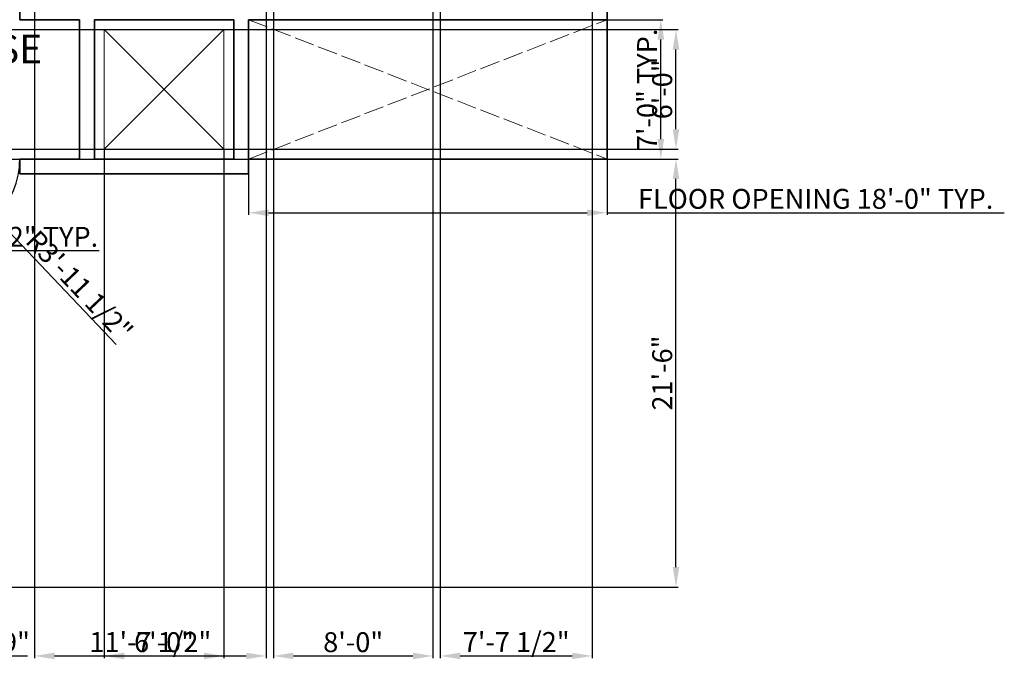
# Model space of a CAD drawing. Units: inches. Extents: x 2174 to 3353, y 1481 to 2316.
# Tile 6 of 8: x 2759 to 3353, y 1501 to 1896. Entities that reach past the tile are written whole.
import ezdxf

# ---------------------------------------------------------------- set-up
doc = ezdxf.new("R2010")
doc.units = ezdxf.units.IN
doc.linetypes.add('ACAD_ISO02W100', pattern=[15, 12, -3])
for name, color, linetype, lineweight in [('A-ANNO-DIMS', 2, 'Continuous', 18), ('A-AREA-IDEN', 7, 'Continuous', 25), ('A-DOOR', 4, 'Continuous', 25), ('A-FLOR-OPEN', 8, 'ACAD_ISO02W100', 13), ('A-FLOR-SHFT', 8, 'Continuous', 18), ('A-WALL', 7, 'Continuous', 35)]:
    doc.layers.add(name, color=color, linetype=linetype, lineweight=lineweight)
doc.styles.get("Standard").update_dxf_attribs({"font": 'arial.ttf'})
doc.dimstyles.new('ISO-25', dxfattribs={"dimtxt": 12, "dimasz": 12, "dimexe": 1.25, "dimexo": 0.625, "dimtad": 1, "dimlunit": 3, "dimtxsty": 'Standard', "dimcen": 2.5, "dimadec": 0, "dimazin": 0, "dimtfac": 1, "dimtmove": 0, "dimatfit": 3, "dimfxl": 1, "dimarcsym": 0})

# ---------------------------------------------------------------- blocks, each defined once
blk = doc.blocks.new('OPENING-CROSS-18FT-7FT')
for p, q in [((0, 0), (216, 84)), ((0, 84), (216, 0))]:
    blk.add_line(p, q)
blk = doc.blocks.new('*D24')
at = {"layer": 'A-ANNO-DIMS', "color": 0, "lineweight": -2, "transparency": 16777216}
for p, q in [((2706.94, 1762.98), (2706.94, 1755.16)), ((2708.94, 1762.98), (2708.94, 1755.16)), ((2694.94, 1756.41), (2682.94, 1756.41)), ((2706.94, 1756.41), (2708.94, 1756.41)), ((2720.94, 1756.41), (2807.34, 1756.41))]:
    blk.add_line(p, q, dxfattribs=at)
at = {"layer": 'A-ANNO-DIMS', "color": 0, "transparency": 16777216}
for points in [[(2694.94, 1758.41), (2694.94, 1754.41), (2706.94, 1756.41)], [(2720.94, 1758.41), (2720.94, 1754.41), (2708.94, 1756.41)]]:
    blk.add_solid(points, dxfattribs=at)
at = {"layer": 'Defpoints', "color": 0, "transparency": 16777216}
for p in [(2706.94, 1763.61), (2708.94, 1763.61), (2708.94, 1756.41)]:
    blk.add_point(p, dxfattribs=at)
at = {"layer": 'A-ANNO-DIMS', "color": 0, "transparency": 16777216, "insert": (2770.14, 1763.16), "char_height": 12, "attachment_point": 5}
blk.add_mtext('0\'-2" TYP.', dxfattribs=at)
blk = doc.blocks.new('*D31')
at = {"layer": 'A-ANNO-DIMS', "color": 0, "lineweight": -2, "transparency": 16777216}
for p, q in [((2916.37, 1919.69), (2916.37, 1908.31)), ((2988.05, 1919.69), (2988.05, 1908.31)), ((2928.37, 1909.56), (2976.05, 1909.56)), ((2988.05, 1909.56), (3211.72, 1909.56))]:
    blk.add_line(p, q, dxfattribs=at)
at = {"layer": 'A-ANNO-DIMS', "color": 0, "transparency": 16777216}
for points in [[(2928.37, 1911.56), (2928.37, 1907.56), (2916.37, 1909.56)], [(2976.05, 1911.56), (2976.05, 1907.56), (2988.05, 1909.56)]]:
    blk.add_solid(points, dxfattribs=at)
at = {"layer": 'Defpoints', "color": 0, "transparency": 16777216}
for p in [(2916.37, 1920.31), (2988.05, 1920.31), (2988.05, 1909.56)]:
    blk.add_point(p, dxfattribs=at)
at = {"layer": 'A-ANNO-DIMS', "color": 0, "transparency": 16777216, "insert": (3105.88, 1916.39), "char_height": 12, "attachment_point": 5}
blk.add_mtext('DINING SET 5\'-11 1/2" TYP.', dxfattribs=at)
blk = doc.blocks.new('*D39')
at = {"layer": 'A-ANNO-DIMS', "color": 0, "lineweight": -2, "transparency": 16777216}
for p, q in [((2897.44, 1810.98), (2897.44, 1777.96)), ((3113.44, 1810.98), (3113.44, 1777.96)), ((2909.44, 1779.21), (3101.44, 1779.21)), ((3113.44, 1779.21), (3352.86, 1779.21))]:
    blk.add_line(p, q, dxfattribs=at)
at = {"layer": 'A-ANNO-DIMS', "color": 0, "transparency": 16777216}
for points in [[(2909.44, 1781.21), (2909.44, 1777.21), (2897.44, 1779.21)], [(3101.44, 1781.21), (3101.44, 1777.21), (3113.44, 1779.21)]]:
    blk.add_solid(points, dxfattribs=at)
at = {"layer": 'Defpoints', "color": 0, "transparency": 16777216}
for p in [(2897.44, 1811.61), (3113.44, 1811.61), (3113.44, 1779.21)]:
    blk.add_point(p, dxfattribs=at)
at = {"layer": 'A-ANNO-DIMS', "color": 0, "transparency": 16777216, "insert": (3239.15, 1786.04), "char_height": 12, "attachment_point": 5}
blk.add_mtext('FLOOR OPENING 18\'-0" TYP.', dxfattribs=at)
blk = doc.blocks.new('*D40')
at = {"layer": 'A-ANNO-DIMS', "color": 0, "lineweight": -2, "transparency": 16777216}
for p, q in [((3114.07, 1895.61), (3147.09, 1895.61)), ((3145.84, 1823.61), (3145.84, 1883.61)), ((3114.07, 1811.61), (3147.09, 1811.61))]:
    blk.add_line(p, q, dxfattribs=at)
at = {"layer": 'A-ANNO-DIMS', "color": 0, "transparency": 16777216}
for points in [[(3143.84, 1883.61), (3147.84, 1883.61), (3145.84, 1895.61)], [(3143.84, 1823.61), (3147.84, 1823.61), (3145.84, 1811.61)]]:
    blk.add_solid(points, dxfattribs=at)
at = {"layer": 'Defpoints', "color": 0, "transparency": 16777216}
for p in [(3113.44, 1895.61), (3145.84, 1895.61), (3113.44, 1811.61)]:
    blk.add_point(p, dxfattribs=at)
at = {"layer": 'A-ANNO-DIMS', "color": 0, "transparency": 16777216, "insert": (3139.09, 1853.61), "char_height": 12, "attachment_point": 5, "rotation": 90}
blk.add_mtext('7\'-0" TYP.', dxfattribs=at)
blk = doc.blocks.new('*D43')
at = {"layer": 'A-ANNO-DIMS', "color": 0, "lineweight": -2, "transparency": 16777216}
for p, q in [((2707.57, 1811.61), (3156.24, 1811.61)), ((3154.99, 1565.61), (3154.99, 1799.61)), ((2707.57, 1553.61), (3156.24, 1553.61))]:
    blk.add_line(p, q, dxfattribs=at)
at = {"layer": 'A-ANNO-DIMS', "color": 0, "transparency": 16777216}
for points in [[(3152.99, 1799.61), (3156.99, 1799.61), (3154.99, 1811.61)], [(3152.99, 1565.61), (3156.99, 1565.61), (3154.99, 1553.61)]]:
    blk.add_solid(points, dxfattribs=at)
at = {"layer": 'Defpoints', "color": 0, "transparency": 16777216}
for p in [(2706.94, 1811.61), (3154.99, 1811.61), (2706.94, 1553.61)]:
    blk.add_point(p, dxfattribs=at)
at = {"layer": 'A-ANNO-DIMS', "color": 0, "transparency": 16777216, "insert": (3148.24, 1682.61), "char_height": 12, "attachment_point": 5, "rotation": 90}
blk.add_mtext('21\'-6"', dxfattribs=at)
blk = doc.blocks.new('*D55')
at = {"layer": 'A-ANNO-DIMS', "color": 0, "lineweight": -2, "transparency": 16777216}
for p, q in [((2768.44, 2143.98), (2768.44, 1510.81)), ((2907.94, 2143.98), (2907.94, 1510.81)), ((2780.44, 1512.06), (2895.94, 1512.06))]:
    blk.add_line(p, q, dxfattribs=at)
at = {"layer": 'A-ANNO-DIMS', "color": 0, "transparency": 16777216}
for points in [[(2780.44, 1514.06), (2780.44, 1510.06), (2768.44, 1512.06)], [(2895.94, 1514.06), (2895.94, 1510.06), (2907.94, 1512.06)]]:
    blk.add_solid(points, dxfattribs=at)
at = {"layer": 'Defpoints', "color": 0, "transparency": 16777216}
for p in [(2768.44, 2144.61), (2907.94, 2144.61), (2907.94, 1512.06)]:
    blk.add_point(p, dxfattribs=at)
at = {"layer": 'A-ANNO-DIMS', "color": 0, "transparency": 16777216, "insert": (2838.19, 1518.89), "char_height": 12, "attachment_point": 5}
blk.add_mtext('11\'-7 1/2"', dxfattribs=at)
blk = doc.blocks.new('*D56')
at = {"layer": 'A-ANNO-DIMS', "color": 0, "lineweight": -2, "transparency": 16777216}
for p, q in [((2912.44, 2143.98), (2912.44, 1510.81)), ((3008.44, 2143.98), (3008.44, 1510.81)), ((2924.44, 1512.06), (2996.44, 1512.06))]:
    blk.add_line(p, q, dxfattribs=at)
at = {"layer": 'A-ANNO-DIMS', "color": 0, "transparency": 16777216}
for points in [[(2924.44, 1514.06), (2924.44, 1510.06), (2912.44, 1512.06)], [(2996.44, 1514.06), (2996.44, 1510.06), (3008.44, 1512.06)]]:
    blk.add_solid(points, dxfattribs=at)
at = {"layer": 'Defpoints', "color": 0, "transparency": 16777216}
for p in [(2912.44, 2144.61), (3008.44, 2144.61), (3008.44, 1512.06)]:
    blk.add_point(p, dxfattribs=at)
at = {"layer": 'A-ANNO-DIMS', "color": 0, "transparency": 16777216, "insert": (2960.44, 1518.81), "char_height": 12, "attachment_point": 5}
blk.add_mtext('8\'-0"', dxfattribs=at)
blk = doc.blocks.new('*D57')
at = {"layer": 'A-ANNO-DIMS', "color": 0, "lineweight": -2, "transparency": 16777216}
for p, q in [((3012.94, 2143.98), (3012.94, 1510.81)), ((3104.44, 2143.98), (3104.44, 1510.81)), ((3024.94, 1512.06), (3092.44, 1512.06))]:
    blk.add_line(p, q, dxfattribs=at)
at = {"layer": 'A-ANNO-DIMS', "color": 0, "transparency": 16777216}
for points in [[(3024.94, 1514.06), (3024.94, 1510.06), (3012.94, 1512.06)], [(3092.44, 1514.06), (3092.44, 1510.06), (3104.44, 1512.06)]]:
    blk.add_solid(points, dxfattribs=at)
at = {"layer": 'Defpoints', "color": 0, "transparency": 16777216}
for p in [(3012.94, 2144.61), (3104.44, 2144.61), (3104.44, 1512.06)]:
    blk.add_point(p, dxfattribs=at)
at = {"layer": 'A-ANNO-DIMS', "color": 0, "transparency": 16777216, "insert": (3058.69, 1518.89), "char_height": 12, "attachment_point": 5}
blk.add_mtext('7\'-7 1/2"', dxfattribs=at)
blk = doc.blocks.new('*D61')
at = {"layer": 'A-ANNO-DIMS', "color": 0, "lineweight": -2, "transparency": 16777216}
for p, q in [((2517.07, 1889.61), (3156.24, 1889.61)), ((3154.99, 1829.61), (3154.99, 1877.61)), ((2517.07, 1817.61), (3156.24, 1817.61))]:
    blk.add_line(p, q, dxfattribs=at)
at = {"layer": 'A-ANNO-DIMS', "color": 0, "transparency": 16777216}
for points in [[(3152.99, 1877.61), (3156.99, 1877.61), (3154.99, 1889.61)], [(3152.99, 1829.61), (3156.99, 1829.61), (3154.99, 1817.61)]]:
    blk.add_solid(points, dxfattribs=at)
at = {"layer": 'Defpoints', "color": 0, "transparency": 16777216}
for p in [(2516.44, 1889.61), (3154.99, 1889.61), (2516.44, 1817.61)]:
    blk.add_point(p, dxfattribs=at)
at = {"layer": 'A-ANNO-DIMS', "color": 0, "transparency": 16777216, "insert": (3148.24, 1853.61), "char_height": 12, "attachment_point": 5, "rotation": 90}
blk.add_mtext('6\'-0"', dxfattribs=at)
blk = doc.blocks.new('*D62')
at = {"layer": 'A-ANNO-DIMS', "color": 0, "lineweight": -2, "transparency": 16777216}
for p, q in [((2810.44, 1816.98), (2810.44, 1510.81)), ((2882.44, 1816.98), (2882.44, 1510.81)), ((2822.44, 1512.06), (2870.44, 1512.06))]:
    blk.add_line(p, q, dxfattribs=at)
at = {"layer": 'A-ANNO-DIMS', "color": 0, "transparency": 16777216}
for points in [[(2822.44, 1514.06), (2822.44, 1510.06), (2810.44, 1512.06)], [(2870.44, 1514.06), (2870.44, 1510.06), (2882.44, 1512.06)]]:
    blk.add_solid(points, dxfattribs=at)
at = {"layer": 'Defpoints', "color": 0, "transparency": 16777216}
for p in [(2810.44, 1817.61), (2882.44, 1817.61), (2882.44, 1512.06)]:
    blk.add_point(p, dxfattribs=at)
at = {"layer": 'A-ANNO-DIMS', "color": 0, "transparency": 16777216, "insert": (2846.44, 1518.81), "char_height": 12, "attachment_point": 5}
blk.add_mtext('6\'-0"', dxfattribs=at)
blk = doc.blocks.new('*D63')
at = {"layer": 'A-ANNO-DIMS', "color": 0, "lineweight": -2, "transparency": 16777216}
for p, q in [((2883.07, 1889.61), (3156.24, 1889.61)), ((3154.99, 1829.61), (3154.99, 1877.61)), ((2883.07, 1817.61), (3156.24, 1817.61))]:
    blk.add_line(p, q, dxfattribs=at)
at = {"layer": 'A-ANNO-DIMS', "color": 0, "transparency": 16777216}
for points in [[(3152.99, 1877.61), (3156.99, 1877.61), (3154.99, 1889.61)], [(3152.99, 1829.61), (3156.99, 1829.61), (3154.99, 1817.61)]]:
    blk.add_solid(points, dxfattribs=at)
at = {"layer": 'Defpoints', "color": 0, "transparency": 16777216}
for p in [(2882.44, 1889.61), (3154.99, 1889.61), (2882.44, 1817.61)]:
    blk.add_point(p, dxfattribs=at)
at = {"layer": 'A-ANNO-DIMS', "color": 0, "transparency": 16777216, "insert": (3148.24, 1853.61), "char_height": 12, "attachment_point": 5, "rotation": 90}
blk.add_mtext('6\'-0"', dxfattribs=at)
blk = doc.blocks.new('*D74')
at = {"layer": 'A-ANNO-DIMS', "color": 0, "lineweight": -2, "transparency": 16777216}
for p, q in [((2697.94, 1561.98), (2697.94, 1510.81)), ((2706.94, 1552.98), (2706.94, 1510.81)), ((2685.94, 1512.06), (2673.94, 1512.06)), ((2697.94, 1512.06), (2706.94, 1512.06)), ((2718.94, 1512.06), (2764.09, 1512.06))]:
    blk.add_line(p, q, dxfattribs=at)
at = {"layer": 'A-ANNO-DIMS', "color": 0, "transparency": 16777216}
for points in [[(2685.94, 1514.06), (2685.94, 1510.06), (2697.94, 1512.06)], [(2718.94, 1514.06), (2718.94, 1510.06), (2706.94, 1512.06)]]:
    blk.add_solid(points, dxfattribs=at)
at = {"layer": 'Defpoints', "color": 0, "transparency": 16777216}
for p in [(2697.94, 1562.61), (2706.94, 1553.61), (2706.94, 1512.06)]:
    blk.add_point(p, dxfattribs=at)
at = {"layer": 'A-ANNO-DIMS', "color": 0, "transparency": 16777216, "insert": (2747.52, 1518.81), "char_height": 12, "attachment_point": 5}
blk.add_mtext('0\'-9"', dxfattribs=at)
blk = doc.blocks.new('*D77')
at = {"layer": 'A-ANNO-DIMS', "color": 0, "lineweight": -2, "transparency": 16777216}
for p, q in [((2711.9, 1811.07), (2744.66, 1776.6)), ((2817.63, 1699.83), (2752.92, 1767.9))]:
    blk.add_line(p, q, dxfattribs=at)
at = {"layer": 'A-ANNO-DIMS', "color": 0, "transparency": 16777216}
blk.add_solid([(2754.37, 1769.28), (2751.47, 1766.52), (2744.66, 1776.6)], dxfattribs=at)
at = {"layer": 'Defpoints', "color": 0, "transparency": 16777216}
for p in [(2711.9, 1811.07), (2744.66, 1776.6)]:
    blk.add_point(p, dxfattribs=at)
at = {"layer": 'A-ANNO-DIMS', "color": 0, "transparency": 16777216, "insert": (2794.36, 1734.22), "char_height": 12, "attachment_point": 5, "rotation": 313.54601}
blk.add_mtext('R3\'-11 1/2"', dxfattribs=at)

msp = doc.modelspace()

# ---------------------------------------------------------------- linework, layer by layer
at = {"layer": 'A-DOOR'}
msp.add_arc((2711.898, 1811.065), 47.549, 266.438577, 0.653632, dxfattribs=at)
at = {"layer": 'A-FLOR-SHFT'}
for p, q in [((2810.444, 1889.608), (2810.444, 1817.608)), ((2810.444, 1889.608), (2882.444, 1889.608)), ((2810.444, 1817.608), (2882.444, 1889.608)), ((2882.444, 1817.608), (2810.444, 1889.608)), ((2882.444, 1889.608), (2882.444, 1817.608)), ((2810.444, 1817.608), (2882.444, 1817.608))]:
    msp.add_line(p, q, dxfattribs=at)
at = {"layer": 'A-WALL'}
for p, q in [((3113.444, 2153.608), (3113.444, 1895.608)), ((2759.444, 2108.608), (2759.444, 1895.608)), ((2759.444, 1895.608), (2795.444, 1895.608)), ((2795.444, 1895.608), (2795.444, 1811.608)), ((2804.444, 1895.608), (2804.444, 1811.608)), ((2804.444, 1895.608), (2888.444, 1895.608)), ((2888.444, 1895.608), (2888.444, 1811.608)), ((2897.444, 1895.608), (2897.444, 1802.608)), ((2897.444, 1895.608), (3113.444, 1895.608)), ((3113.444, 1811.608), (3113.444, 1895.608)), ((2759.444, 1811.608), (2759.444, 1802.608)), ((2759.444, 1811.608), (2795.444, 1811.608)), ((2804.444, 1811.608), (2888.444, 1811.608)), ((2897.444, 1811.608), (3113.444, 1811.608)), ((2759.444, 1802.608), (2897.444, 1802.608))]:
    msp.add_line(p, q, dxfattribs=at)

# ---------------------------------------------------------------- block references
at = {"layer": 'A-FLOR-OPEN'}
msp.add_blockref('OPENING-CROSS-18FT-7FT', (2897.444, 1811.608), dxfattribs=at)

# ---------------------------------------------------------------- texts
at = {"layer": 'A-AREA-IDEN', "insert": (2645.911, 1886.581), "char_height": 17.3039, "attachment_point": 1}
msp.add_mtext_dynamic_manual_height_columns('STAIR CASE', width=375.7284, gutter_width=86.519, heights=[0], dxfattribs=at)

# ---------------------------------------------------------------- dimensions: what is measured, and where the dimension line sits
at = {"layer": 'A-ANNO-DIMS'}
for base, p1, p2, picture, middle in [((2907.944, 1512.058), (2768.444, 2144.608), (2907.944, 2144.608), '*D55', (2838.194, 1518.887)), ((3008.444, 1512.058), (2912.444, 2144.608), (3008.444, 2144.608), '*D56', (2960.444, 1518.809)), ((3104.444, 1512.058), (3012.944, 2144.608), (3104.444, 2144.608), '*D57', (3058.694, 1518.887)), ((2882.444, 1512.058), (2810.444, 1817.608), (2882.444, 1817.608), '*D62', (2846.444, 1518.809)), ((2706.944, 1512.058), (2697.944, 1562.608), (2706.944, 1553.608), '*D74', (2747.519, 1518.809))]:
    dim = msp.add_linear_dim(base=base, p1=p1, p2=p2, dimstyle='ISO-25', override={"dimdec": 1, "dimlfac": 1, "dimrnd": 0, "dimzin": 1, "dimdsep": 46, "dimlunit": 4, "dimfrac": 2}, dxfattribs=at)
    dim.commit()
    dim.dimension.update_dxf_attribs({"geometry": picture, "text_midpoint": middle})
for base, p1, p2, text, picture, middle in [((2988.046, 1909.562), (2916.374, 1920.313), (2988.046, 1920.313), 'DINING SET <> TYP.', '*D31', (3105.884, 1916.392)), ((3113.444, 1779.208), (2897.444, 1811.608), (3113.444, 1811.608), 'FLOOR OPENING <> TYP.', '*D39', (3239.153, 1786.041)), ((2708.944, 1756.408), (2706.944, 1763.608), (2708.944, 1763.608), '<> TYP.', '*D24', (2770.142, 1763.159))]:
    dim = msp.add_linear_dim(base=base, p1=p1, p2=p2, text=text, dimstyle='ISO-25', override={"dimdec": 1, "dimlfac": 1, "dimrnd": 0, "dimzin": 1, "dimdsep": 46, "dimlunit": 4, "dimfrac": 2}, dxfattribs=at)
    dim.commit()
    dim.dimension.update_dxf_attribs({"geometry": picture, "text_midpoint": middle})
dim = msp.add_linear_dim(base=(3145.844, 1895.608), p1=(3113.444, 1811.608), p2=(3113.444, 1895.608), angle=90, text='<> TYP.', dimstyle='ISO-25', override={"dimdec": 1, "dimlfac": 1, "dimrnd": 0, "dimzin": 1, "dimdsep": 46, "dimlunit": 4, "dimfrac": 2}, dxfattribs=at)
dim.commit()
dim.dimension.update_dxf_attribs({"geometry": '*D40', "text_midpoint": (3139.093, 1853.608)})
for base, p1, p2, picture, middle in [((3154.994, 1889.608), (2516.444, 1817.608), (2516.444, 1889.608), '*D61', (3148.243, 1853.608)), ((3154.994, 1889.608), (2882.444, 1817.608), (2882.444, 1889.608), '*D63', (3148.243, 1853.608)), ((3154.994, 1811.608), (2706.944, 1553.608), (2706.944, 1811.608), '*D43', (3148.243, 1682.608))]:
    dim = msp.add_linear_dim(base=base, p1=p1, p2=p2, angle=90, dimstyle='ISO-25', override={"dimdec": 1, "dimlfac": 1, "dimrnd": 0, "dimzin": 1, "dimdsep": 46, "dimlunit": 4, "dimfrac": 2}, dxfattribs=at)
    dim.commit()
    dim.dimension.update_dxf_attribs({"geometry": picture, "text_midpoint": middle})
dim = msp.add_radius_dim(center=(2711.898, 1811.065), mpoint=(2744.657, 1776.6), dimstyle='ISO-25', override={"dimdec": 1, "dimlfac": 1, "dimrnd": 0, "dimzin": 1, "dimdsep": 46, "dimlunit": 4, "dimfrac": 2}, dxfattribs=at)
dim.commit()
dim.dimension.update_dxf_attribs({"geometry": '*D77', "text_midpoint": (2794.363, 1734.225)})

doc.saveas('drawing.dxf')
